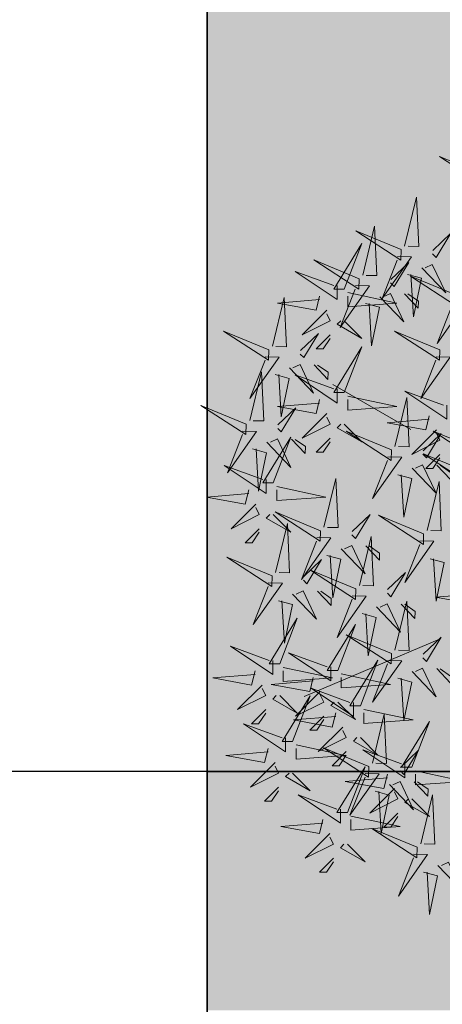
# Model space of a CAD drawing. Units: inches. Extents: x 1704 to 6393, y -157 to 1172.
# Tile 54 of 122: x 1892 to 1906, y 887 to 920. Entities that reach past the tile are written whole.
import ezdxf

# ---------------------------------------------------------------- set-up
doc = ezdxf.new("R2010")
doc.units = ezdxf.units.IN
doc.header["$MEASUREMENT"] = 0
for name, color, linetype, lineweight in [('A-ANNO-DIMS', 7, 'Continuous', 13), ('C-PROP', 7, 'Continuous', 35), ('L-shrub', 74, 'Continuous', 18), ('WALLS', 7, 'Continuous', 35)]:
    doc.layers.add(name, color=color, linetype=linetype, lineweight=lineweight)
doc.layers.add('L-HRDS-PATT', color=9, linetype='Continuous', lineweight=13, true_color=0xc5c1ba)
doc.styles.get("Standard").update_dxf_attribs({"font": 'arial.ttf'})
doc.dimstyles.get("Standard").update_dxf_attribs({"dimtxt": 6, "dimasz": 2, "dimexe": 0.18, "dimexo": 0.0625, "dimgap": 0.09, "dimtad": 0, "dimtih": 1, "dimtoh": 1, "dimdec": 1, "dimzin": 0, "dimdsep": 46, "dimlunit": 3, "dimtxsty": 'Standard', "dimblk": 'ARCHTICK', "dimcen": 0.09, "dimadec": 0, "dimazin": 0, "dimtfac": 1, "dimtdec": 1, "dimtofl": 0, "dimtmove": 0, "dimatfit": 3, "dimfxl": 1, "dimtolj": 1, "dimtzin": 0, "dimarcsym": 0})

# ---------------------------------------------------------------- blocks, each defined once
blk = doc.blocks.new('shrub3')
for p, q in [((-68.47, 143.52), (-106.19, 232.32)), ((68.94, 162.35), (98.58, 213.48))]:
    blk.add_line(p, q)
for points in [[(72.58, 270.39), (84.86, 300.11), (65.67, 270.57), (72.58, 270.39)], [(-89.4, 264.53), (-98.64, 266.83), (-94.02, 292.2), (-91.71, 264.53)], [(29.32, 268.76), (20.08, 271.07), (24.7, 296.43), (27.01, 268.76)], [(36.24, 257.23), (27.01, 257.23), (45.48, 284.9), (36.24, 259.54)], [(121.34, 255.57), (133.62, 285.29), (114.43, 255.75), (121.34, 255.57)], [(-140.28, 256.06), (-149.52, 258.36), (-144.9, 283.73), (-142.59, 256.06)], [(-82.48, 253), (-91.71, 253), (-73.24, 280.67), (-82.48, 255.31)], [(-27.06, 253.45), (-14.78, 283.17), (-33.97, 253.63), (-27.06, 253.45)], [(20.08, 264.15), (3.92, 280.29), (13.16, 261.85), (17.78, 264.15)], [(68.03, 272.82), (67.8, 263.59), (40.6, 282.74), (65.73, 272.87)], [(-133.36, 244.53), (-142.59, 244.53), (-124.12, 272.2), (-133.36, 246.84)], [(-98.64, 259.92), (-114.8, 276.06), (-105.56, 257.61), (-100.94, 259.92)], [(-149.52, 251.45), (-165.68, 267.59), (-156.44, 249.14), (-151.83, 251.45)], [(-114.8, 257.61), (-124.03, 266.83), (-124.03, 262.22), (-117.11, 257.61)], [(-31.61, 255.88), (-31.84, 246.65), (-59.04, 265.8), (-33.91, 255.94)], [(3.92, 261.85), (-5.31, 271.07), (-5.31, 266.46), (1.62, 261.85)], [(56.33, 266.18), (53.8, 257.01), (28.56, 262.26), (56.27, 263.87)], [(74.83, 268.03), (106.93, 260.3), (74.6, 258.8), (74.77, 265.72)], [(116.79, 258), (116.56, 248.76), (89.36, 267.92), (114.49, 258.05)], [(33.94, 252.62), (63.95, 241.09), (33.94, 259.54), (33.94, 252.62)], [(-165.68, 249.14), (-174.91, 258.36), (-174.91, 253.75), (-167.99, 249.14)], [(-105.56, 248.39), (-117.11, 236.86), (-107.87, 253), (-105.56, 250.69)], [(-93.64, 226.42), (-102.88, 228.72), (-98.26, 254.08), (-95.95, 226.42)], [(-84.78, 248.39), (-54.77, 236.86), (-84.78, 255.31), (-84.78, 248.39)], [(13.16, 252.62), (1.62, 241.09), (10.85, 257.23), (13.16, 254.93)], [(60.71, 256.84), (44.17, 241.08), (62.84, 249.85), (60.65, 254.53)], [(123.59, 253.21), (155.69, 245.48), (123.36, 243.97), (123.53, 250.9)], [(-186.92, 220.06), (-196.16, 222.37), (-191.54, 247.73), (-189.23, 220.06)], [(-135.66, 239.92), (-105.65, 228.39), (-135.66, 246.84), (-135.66, 239.92)], [(-87.09, 246.08), (-94.02, 213.8), (-96.33, 246.08), (-89.4, 246.08)], [(-43.31, 249.24), (-45.84, 240.07), (-71.08, 245.32), (-43.37, 246.93)], [(-24.81, 251.09), (7.29, 243.36), (-25.04, 241.86), (-24.87, 248.78)], [(2.62, 221.69), (14.9, 251.41), (-4.29, 221.87), (2.62, 221.69)], [(31.63, 250.32), (24.7, 218.04), (22.39, 250.32), (29.32, 250.32)], [(72.06, 249.62), (83.3, 237.79), (67.4, 247.43), (69.76, 249.68)], [(105.09, 251.36), (102.56, 242.19), (77.32, 247.44), (105.04, 249.05)], [(88.68, 222.18), (79.44, 224.49), (84.06, 249.85), (86.37, 222.18)], [(156.52, 222.18), (147.29, 224.49), (151.9, 249.85), (154.21, 222.18)], [(-156.44, 239.92), (-167.99, 228.39), (-158.75, 244.53), (-156.44, 242.22)], [(-116.96, 211.59), (-126.2, 213.9), (-121.58, 239.26), (-119.27, 211.59)], [(-86.72, 214.89), (-95.95, 214.89), (-77.48, 242.56), (-86.72, 217.19)], [(-38.93, 239.9), (-55.47, 224.14), (-36.8, 232.91), (-38.99, 237.59)], [(62.61, 240.62), (53.16, 231.62), (57.77, 231.51), (62.55, 238.31)], [(109.47, 242.01), (92.93, 226.26), (111.6, 235.03), (109.41, 239.71)], [(-180, 208.53), (-189.23, 208.53), (-170.76, 236.2), (-180, 210.84)], [(-137.97, 237.61), (-144.9, 205.33), (-147.21, 237.61), (-140.28, 237.61)], [(-102.88, 221.8), (-119.04, 237.94), (-109.8, 219.5), (-105.18, 221.8)], [(-27.58, 232.68), (-16.34, 220.86), (-32.24, 230.49), (-29.88, 232.74)], [(-1.93, 224.12), (-2.16, 214.89), (-29.36, 234.04), (-4.23, 224.17)], [(79.44, 217.57), (63.28, 233.71), (72.52, 215.26), (77.14, 217.57)], [(95.61, 210.65), (86.37, 210.65), (104.84, 238.32), (95.61, 212.96)], [(120.82, 234.8), (132.06, 222.97), (116.16, 232.61), (118.52, 234.86)], [(147.29, 217.57), (131.13, 233.71), (140.36, 215.26), (144.98, 217.57)], [(163.45, 210.65), (154.21, 210.65), (172.68, 238.32), (163.45, 212.96)], [(-196.16, 215.45), (-212.32, 231.59), (-203.08, 213.15), (-198.47, 215.45)], [(-119.04, 219.5), (-128.27, 228.72), (-128.27, 224.11), (-121.35, 219.5)], [(-110.04, 200.06), (-119.27, 200.06), (-100.8, 227.73), (-110.04, 202.37)], [(-35.54, 198.4), (-23.26, 228.12), (-42.45, 198.58), (-35.54, 198.4)], [(-212.32, 213.15), (-221.55, 222.37), (-221.55, 217.76), (-214.63, 213.15)], [(-126.2, 206.98), (-142.36, 223.12), (-133.12, 204.68), (-128.5, 206.98)], [(-37.03, 223.68), (-46.48, 214.68), (-41.87, 214.57), (-37.09, 221.37)], [(63.28, 215.26), (54.05, 224.49), (54.05, 219.87), (60.98, 215.26)], [(111.37, 225.8), (101.92, 216.8), (106.53, 216.68), (111.31, 223.49)], [(131.13, 215.26), (121.89, 224.49), (121.89, 219.87), (128.82, 215.26)], [(167.98, 196.29), (180.26, 226), (161.07, 196.46), (167.98, 196.29)], [(-152.14, 189.93), (-139.86, 219.65), (-159.05, 190.11), (-152.14, 189.93)], [(-142.36, 204.68), (-151.59, 213.9), (-151.59, 209.29), (-144.67, 204.68)], [(-109.8, 210.27), (-121.35, 198.75), (-112.11, 214.89), (-109.8, 212.58)], [(-89.02, 210.27), (-59.01, 198.75), (-89.02, 217.19), (-89.02, 210.27)], [(-13.63, 217.48), (-16.16, 208.31), (-41.4, 213.56), (-13.69, 215.17)], [(4.87, 219.33), (36.97, 211.6), (4.64, 210.1), (4.81, 217.02)], [(-203.08, 203.92), (-214.63, 192.39), (-205.39, 208.53), (-203.08, 206.23)], [(-182.31, 203.92), (-152.29, 192.39), (-182.31, 210.84), (-182.31, 203.92)], [(-91.33, 207.97), (-98.26, 175.69), (-100.57, 207.97), (-93.64, 207.97)], [(-40.09, 200.83), (-40.32, 191.59), (-67.52, 210.75), (-42.39, 200.88)], [(-9.25, 208.13), (-25.79, 192.38), (-7.12, 201.15), (-9.31, 205.83)], [(72.52, 206.04), (60.98, 194.51), (70.21, 210.65), (72.52, 208.35)], [(93.3, 206.04), (123.31, 194.51), (93.3, 212.96), (93.3, 206.04)], [(140.36, 206.04), (128.82, 194.51), (138.05, 210.65), (140.36, 208.35)], [(163.43, 198.71), (163.2, 189.48), (136, 208.63), (161.13, 198.77)], [(161.14, 206.04), (191.15, 194.51), (161.14, 212.96), (161.14, 206.04)], [(-184.61, 201.62), (-191.54, 169.34), (-193.85, 201.62), (-186.92, 201.62)], [(-156.69, 192.36), (-156.92, 183.12), (-184.12, 202.28), (-159, 192.41)], [(-157.24, 177.72), (-166.48, 180.02), (-161.86, 205.38), (-159.55, 177.72)], [(-112.34, 195.45), (-82.33, 183.92), (-112.34, 202.37), (-112.34, 195.45)], [(-77.94, 175.11), (-65.66, 204.83), (-84.85, 175.28), (-77.94, 175.11)], [(2.1, 200.92), (13.34, 189.09), (-2.56, 198.73), (-0.2, 200.98)], [(55.62, 175.11), (67.9, 204.83), (48.71, 175.28), (55.62, 175.11)], [(90.99, 203.73), (84.06, 171.45), (81.75, 203.73), (88.68, 203.73)], [(158.83, 203.73), (151.9, 171.45), (149.59, 203.73), (156.52, 203.73)], [(-150.32, 166.19), (-159.55, 166.19), (-141.08, 193.86), (-150.32, 168.49)], [(-133.12, 195.45), (-144.67, 183.92), (-135.43, 200.06), (-133.12, 197.76)], [(-51.79, 194.19), (-54.32, 185.02), (-79.56, 190.27), (-51.85, 191.88)], [(-33.29, 196.04), (-1.19, 188.31), (-33.52, 186.81), (-33.35, 193.73)], [(170.23, 193.92), (202.33, 186.19), (170, 184.69), (170.17, 191.61)], [(187.06, 168.76), (199.34, 198.47), (180.15, 168.93), (187.06, 168.76)], [(-205.14, 158.17), (-192.86, 187.89), (-212.05, 158.35), (-205.14, 158.17)], [(-166.48, 173.1), (-182.64, 189.24), (-173.4, 170.8), (-168.79, 173.1)], [(-149.89, 187.57), (-117.79, 179.84), (-150.12, 178.34), (-149.95, 185.26)], [(-114.65, 193.15), (-121.58, 160.87), (-123.89, 193.15), (-116.96, 193.15)], [(-82.49, 177.53), (-82.72, 168.3), (-109.92, 187.46), (-84.79, 177.59)], [(-7.35, 191.92), (-16.8, 182.92), (-12.19, 182.81), (-7.41, 189.61)], [(51.07, 177.53), (50.84, 168.3), (23.64, 187.46), (48.77, 177.59)], [(151.73, 192.07), (149.2, 182.9), (123.96, 188.15), (151.68, 189.77)], [(-168.39, 185.72), (-170.92, 176.55), (-196.16, 181.8), (-168.45, 183.41)], [(-47.41, 184.84), (-63.95, 169.09), (-45.28, 177.86), (-47.47, 182.54)], [(0.5, 153.94), (12.78, 183.65), (-6.41, 154.11), (0.5, 153.94)], [(156.11, 182.73), (139.57, 166.97), (158.24, 175.74), (156.05, 180.42)], [(182.51, 171.18), (182.28, 161.95), (155.08, 181.11), (180.21, 171.24)], [(-182.64, 170.8), (-191.87, 180.02), (-191.87, 175.41), (-184.95, 170.8)], [(-164.01, 176.37), (-180.55, 160.62), (-161.88, 169.39), (-164.07, 174.07)], [(-36.06, 177.63), (-24.82, 165.8), (-40.72, 175.44), (-38.36, 177.69)], [(78.08, 150.19), (68.84, 152.49), (73.46, 177.86), (75.77, 150.19)], [(167.46, 175.51), (178.7, 163.69), (162.8, 173.32), (165.16, 175.57)], [(-209.69, 160.6), (-209.92, 151.36), (-237.12, 170.52), (-212, 160.65)], [(-152.66, 169.16), (-141.42, 157.33), (-157.33, 166.97), (-154.96, 169.22)], [(-152.62, 161.57), (-122.61, 150.05), (-152.62, 168.49), (-152.62, 161.57)], [(-94.19, 170.9), (-96.72, 161.73), (-121.96, 166.98), (-94.25, 168.59)], [(-75.69, 172.75), (-43.59, 165.01), (-75.92, 163.51), (-75.75, 170.44)], [(-45.51, 168.63), (-54.96, 159.63), (-50.35, 159.51), (-45.57, 166.32)], [(39.37, 170.9), (36.84, 161.73), (11.6, 166.98), (39.31, 168.59)], [(57.87, 172.75), (89.97, 165.01), (57.64, 163.51), (57.81, 170.44)], [(121.34, 143.35), (133.62, 173.06), (114.43, 143.52), (121.34, 143.35)], [(-173.4, 161.57), (-184.95, 150.05), (-175.71, 166.19), (-173.4, 163.88)], [(-89.81, 161.55), (-106.35, 145.8), (-87.68, 154.57), (-89.87, 159.24)], [(-4.05, 156.36), (-4.28, 147.13), (-31.48, 166.28), (-6.35, 156.42)], [(43.75, 161.55), (27.21, 145.8), (45.88, 154.57), (43.69, 159.24)], [(68.84, 145.58), (52.68, 161.72), (61.92, 143.27), (66.54, 145.58)], [(85.01, 138.66), (75.77, 138.66), (94.24, 166.33), (85.01, 140.97)], [(170.81, 164.55), (168.28, 155.37), (143.04, 160.62), (170.76, 162.24)], [(158.01, 166.51), (148.56, 157.51), (153.17, 157.4), (157.96, 164.21)], [(157.38, 132.76), (169.66, 162.48), (150.47, 132.94), (157.38, 132.76)], [(189.31, 166.39), (221.41, 158.66), (189.08, 157.16), (189.25, 164.09)], [(-202.89, 155.81), (-170.79, 148.07), (-203.12, 146.57), (-202.95, 153.5)], [(-162.11, 160.16), (-171.56, 151.16), (-166.95, 151.04), (-162.17, 157.85)], [(-154.93, 159.27), (-161.86, 126.99), (-164.17, 159.27), (-157.24, 159.27)], [(116.79, 145.77), (116.56, 136.54), (89.36, 155.7), (114.49, 145.83)], [(175.19, 155.2), (158.65, 139.45), (177.32, 148.22), (175.13, 152.89)], [(-221.39, 153.96), (-223.93, 144.79), (-249.17, 150.04), (-221.45, 151.65)], [(-78.46, 154.34), (-67.22, 142.51), (-83.13, 152.15), (-80.76, 154.4)], [(-15.75, 149.73), (-18.28, 140.55), (-43.52, 145.8), (-15.81, 147.42)], [(2.75, 151.57), (34.85, 143.84), (2.52, 142.34), (2.69, 149.26)], [(40.78, 124.29), (53.06, 154.01), (33.87, 124.47), (40.78, 124.29)], [(52.68, 143.27), (43.45, 152.49), (43.45, 147.88), (50.38, 143.27)], [(55.1, 154.34), (66.34, 142.51), (50.44, 152.15), (52.8, 154.4)], [(-217.01, 144.61), (-233.55, 128.86), (-214.88, 137.63), (-217.07, 142.31)], [(-87.91, 145.34), (-97.36, 136.34), (-92.75, 136.22), (-87.97, 143.03)], [(-36.4, 118.43), (-45.64, 120.73), (-41.02, 146.1), (-38.71, 118.43)], [(45.65, 145.34), (36.2, 136.34), (40.81, 136.22), (45.59, 143.03)], [(55.62, 117.94), (67.9, 147.66), (48.71, 118.11), (55.62, 117.94)], [(152.83, 135.19), (152.6, 125.95), (125.4, 145.11), (150.53, 135.24)], [(186.54, 147.99), (197.78, 136.16), (181.88, 145.8), (184.24, 148.05)], [(235.82, 113.71), (248.1, 143.42), (228.91, 113.88), (235.82, 113.71)]]:
    blk.add_lwpolyline(points)
blk = doc.blocks.new('_ArchTick')
at = {"color": 0, "linetype": 'ByBlock', "const_width": 0.15}
blk.add_lwpolyline([(-0.5, -0.5), (0.5, 0.5)], dxfattribs=at)
blk = doc.blocks.new('*D93')
at = {"layer": 'A-ANNO-DIMS', "color": 0, "lineweight": -2, "transparency": 16777216}
for p, q in [((2605.286, 895.213), (1829.698, 895.213)), ((1829.878, 895.213), (1829.878, 495.866)), ((1829.878, 90.213), (1829.878, 489.56)), ((2605.286, 90.213), (1829.698, 90.213))]:
    blk.add_line(p, q, dxfattribs=at)
at = {"layer": 'Defpoints', "color": 0, "lineweight": -3, "transparency": 16777216}
for p in [(2605.349, 895.213), (1829.878, 90.213), (2605.349, 90.213)]:
    blk.add_point(p, dxfattribs=at)
at = {"layer": 'A-ANNO-DIMS', "color": 0, "lineweight": -2, "transparency": 16777216, "xscale": 2, "yscale": 2, "zscale": 2}
for p, rotation in [((1829.878, 895.213), 90), ((1829.878, 90.213), 270)]:
    blk.add_blockref('_ArchTick', p, dxfattribs=dict(at, rotation=rotation))
at = {"layer": 'A-ANNO-DIMS', "color": 0, "transparency": 16777216, "insert": (1829.878, 492.713), "char_height": 6, "attachment_point": 5}
blk.add_mtext('\\A1;805', dxfattribs=at)
blk = doc.blocks.new('*D94')
at = {"layer": 'A-ANNO-DIMS', "color": 0, "lineweight": -2, "transparency": 16777216}
for p, q in [((1898.349, 895.275), (1898.349, 1105.287)), ((1898.349, 1105.107), (1979.39, 1105.107)), ((2073.349, 1105.107), (1992.307, 1105.107)), ((2073.349, 895.275), (2073.349, 1105.287))]:
    blk.add_line(p, q, dxfattribs=at)
at = {"layer": 'Defpoints', "color": 0, "lineweight": -3, "transparency": 16777216}
for p in [(2073.349, 1105.107), (1898.349, 895.213), (2073.349, 895.213)]:
    blk.add_point(p, dxfattribs=at)
at = {"layer": 'A-ANNO-DIMS', "color": 0, "lineweight": -2, "transparency": 16777216, "xscale": 2, "yscale": 2, "zscale": 2, "rotation": 180}
blk.add_blockref('_ArchTick', (1898.349, 1105.107), dxfattribs=at)
at = {"layer": 'A-ANNO-DIMS', "color": 0, "lineweight": -2, "transparency": 16777216, "xscale": 2, "yscale": 2, "zscale": 2}
blk.add_blockref('_ArchTick', (2073.349, 1105.107), dxfattribs=at)
at = {"layer": 'A-ANNO-DIMS', "color": 0, "transparency": 16777216, "insert": (1985.849, 1105.107), "char_height": 6, "attachment_point": 5}
blk.add_mtext('\\A1;175', dxfattribs=at)

msp = doc.modelspace()

# ---------------------------------------------------------------- hatches: boundary and pattern name
at = {"layer": 'L-HRDS-PATT', "transparency": 33554643}
h = msp.add_hatch(color=256, dxfattribs=at)
h.dxf.hatch_style = 1
h.paths.add_polyline_path([(2065.589, 1033.213), (1898.349, 1033.213), (1898.349, 895.213), (2065.589, 895.213)])
h = msp.add_hatch(color=256, dxfattribs=at)
h.dxf.hatch_style = 1
h.paths.add_polyline_path([(2073.349, 719.213), (2021.151, 719.213), (2021.151, 711.213), (2073.349, 711.213)])
h.paths.add_polyline_path([(1977.349, 719.213), (1969.349, 719.213), (1898.349, 719.213), (1898.349, 711.213), (1977.349, 711.213)])
h.paths.add_polyline_path([(1977.349, 895.213), (1898.349, 895.213), (1898.349, 887.213), (1969.349, 887.213), (1977.349, 887.213)])

# ---------------------------------------------------------------- linework, layer by layer
at = {"layer": 'C-PROP'}
msp.add_line((1898.349, -3.787), (1898.349, 1033.213), dxfattribs=at)
at = {"layer": 'WALLS'}
msp.add_line((2167.349, 895.213), (1898.349, 895.213), dxfattribs=at)

# ---------------------------------------------------------------- block references
at = {"layer": 'L-shrub', "xscale": 0.0510581485411622, "yscale": 0.0510581485411622, "zscale": 0.0510581485411622, "rotation": 89.99999999999996}
msp.add_blockref('shrub3', (1913.464, 903.144), dxfattribs=at)

# ---------------------------------------------------------------- dimensions: what is measured, and where the dimension line sits
at = {"layer": 'A-ANNO-DIMS'}
dim = msp.add_linear_dim(base=(2073.349, 1105.107), p1=(1898.349, 895.213), p2=(2073.349, 895.213), dimstyle='Standard', override={"dimdec": 0, "dimlfac": 1, "dimrnd": 0, "dimzin": 0, "dimdsep": 46, "dimlunit": 2}, dxfattribs=at)
dim.commit()
dim.dimension.update_dxf_attribs({"geometry": '*D94', "text_midpoint": (1985.849, 1105.107)})
dim = msp.add_linear_dim(base=(1829.878, 90.213), p1=(2605.349, 895.213), p2=(2605.349, 90.213), angle=90, dimstyle='Standard', override={"dimdec": 0, "dimlfac": 1, "dimrnd": 0, "dimzin": 0, "dimdsep": 46, "dimlunit": 2}, dxfattribs=at)
dim.commit()
dim.dimension.update_dxf_attribs({"geometry": '*D93', "text_midpoint": (1829.878, 492.713)})

doc.saveas('drawing.dxf')
